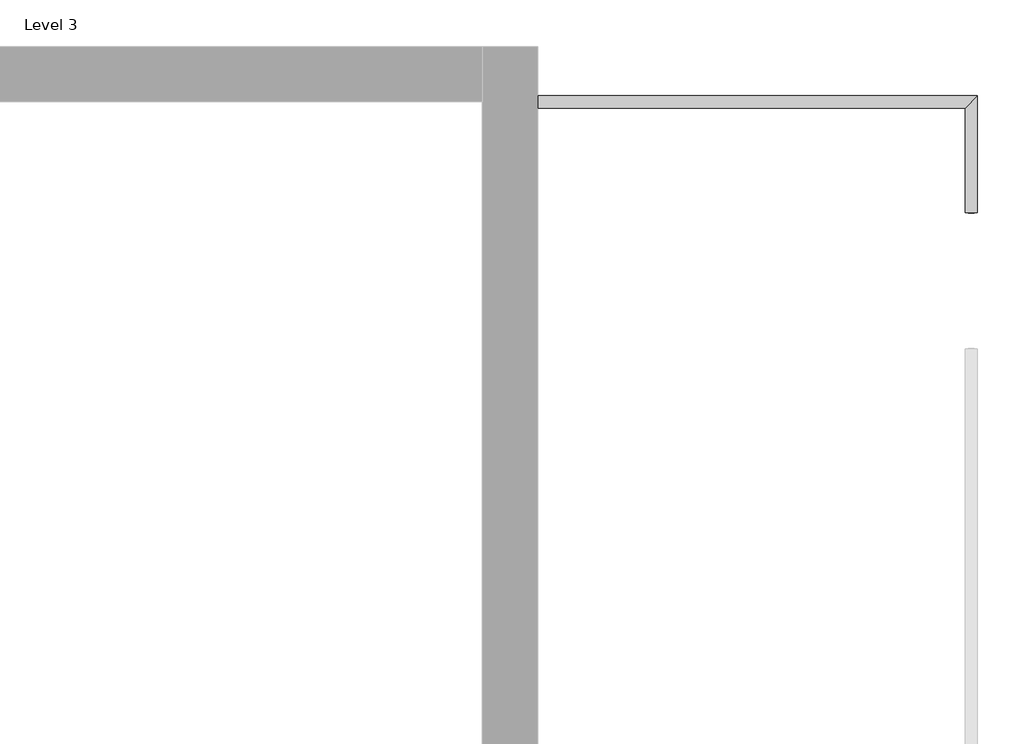
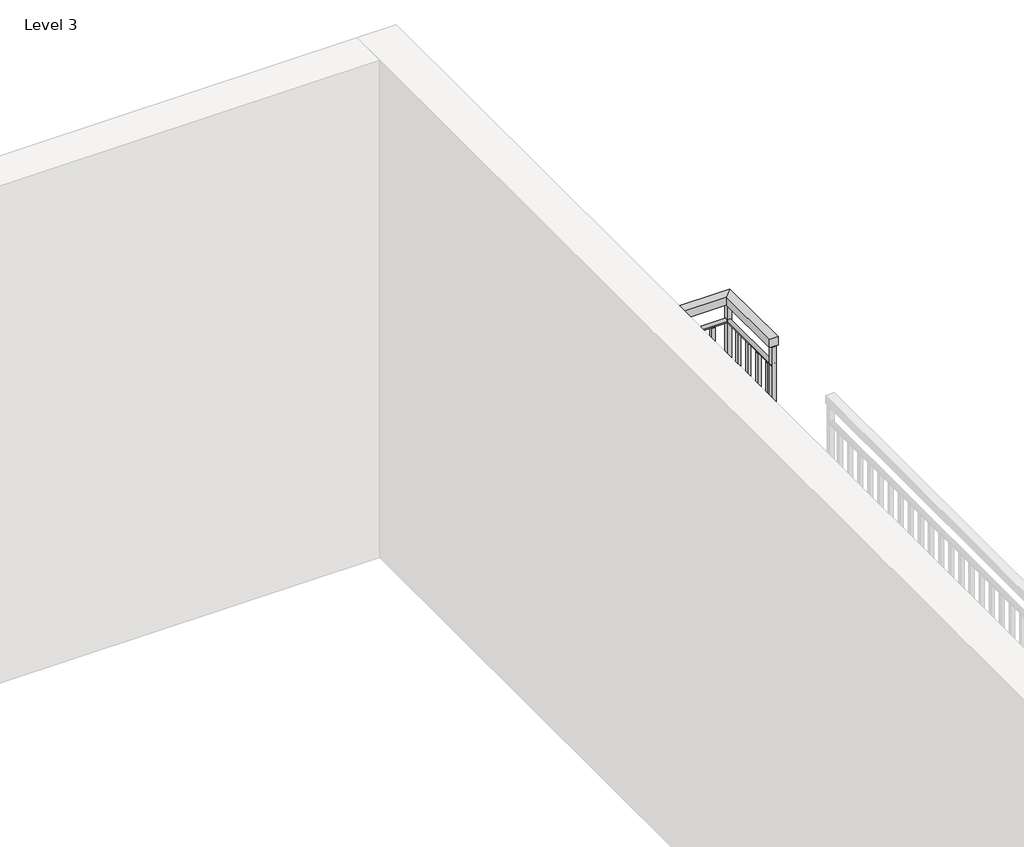
# One storey, part 4 of 4: 1 railing.
"""IFC4 building model written with IfcOpenShell, lengths in millimetres."""

from ifc_helpers import new_model, si_unit, frame, origin, place, context, project, spatial, polyline, circle_curve, ellipse_curve, outline, extrude, faceted_brep, element, save
from ifc_brep_helpers import plane_surface, cylinder_surface, advanced_brep

model = new_model("IFC4")

# Units and contexts
model_context = context("Model", 3, world=origin())
ifc_project = project(units=[si_unit("LENGTHUNIT", "METRE", prefix="MILLI")], contexts=[model_context])

# Site, building, storey
site = spatial("IfcSite", under=ifc_project)
building = spatial("IfcBuilding", under=site)
storey = spatial("IfcBuildingStorey", under=building, Name="Level 3", Elevation=3810.0)

# Railing
placement = place(None, origin())
element("IfcRailing", 1, ObjectType="Handrail - Rectangular", at=placement, inside=storey, context=model_context, shape_type="SolidModel", body=[
    faceted_brep([(6670.6750735, 9193.6050084, 4724.4), (6670.6750735, 9193.6050084, 4673.6), (6670.6750735, 9142.8050084, 4673.6), (6670.6750735, 9142.8050084, 4724.4), (8513.4425759, 9193.6050084, 4724.4), (8513.4425759, 9193.6050084, 4673.6), (8462.6425759, 9142.8050084, 4673.6), (8462.6425759, 9142.8050084, 4724.4), (8513.4425759, 8711.0050084, 4724.4), (8462.6425759, 8711.0050084, 4724.4), (8462.6425759, 8711.0050084, 4673.6), (8513.4425759, 8711.0050084, 4673.6)], [[[0, 1, 2, 3]], [[1, 0, 4, 5]], [[2, 1, 5, 6]], [[3, 2, 6, 7]], [[0, 3, 7, 4]], [[8, 9, 10, 11]], [[5, 4, 8, 11]], [[6, 5, 11, 10]], [[7, 6, 10, 9]], [[4, 7, 9, 8]]]),
    advanced_brep(
    [(6670.6750735, 9180.9050084, 4559.3), (6670.6750735, 9155.5050084, 4559.3), (8500.7425759, 9180.9050084, 4559.3), (8475.3425759, 9155.5050084, 4559.3), (8500.7425759, 8711.0050084, 4559.3), (8475.3425759, 8711.0050084, 4559.3)],
    [
        (0, 1, circle_curve(frame((6670.6750735, 9168.2050084, 4559.3), z_axis=(-1.0, 0.0, 0.0), x_axis=(0.0, -1.0, 0.0)), 12.7)),
        (1, 0, circle_curve(frame((6670.6750735, 9168.2050084, 4559.3), z_axis=(-1.0, 0.0, 0.0), x_axis=(0.0, -1.0, 0.0)), 12.7)),
        (0, 2),
        (2, 3, ellipse_curve(frame((8488.0425759, 9168.2050084, 4559.3), z_axis=(-0.7071067811865466, 0.7071067811865483, 0.0), x_axis=(-0.7071067811865486, -0.7071067811865466, 0.0)), 17.9605122, 12.7)),
        (3, 1),
        (3, 2, ellipse_curve(frame((8488.0425759, 9168.2050084, 4559.3), z_axis=(-0.7071067811865466, 0.7071067811865483, 0.0), x_axis=(-0.7071067811865486, -0.7071067811865466, 0.0)), 17.9605122, 12.7)),
        (4, 5, circle_curve(frame((8488.0425759, 8711.0050084, 4559.3), z_axis=(0.0, -1.0, 0.0), x_axis=(-1.0, 0.0, 0.0)), 12.7)),
        (5, 4, circle_curve(frame((8488.0425759, 8711.0050084, 4559.3), z_axis=(0.0, -1.0, 0.0), x_axis=(-1.0, 0.0, 0.0)), 12.7)),
        (2, 4),
        (5, 3),
    ],
    [
        plane_surface(frame((6670.6750735, 9168.2050084, 4572.0), z_axis=(-1.0, 0.0, 0.0), x_axis=(0.0, 1.0, 0.0))),
        cylinder_surface(frame((6670.6750735, 9168.2050084, 4559.3), z_axis=(-1.0, 0.0, 0.0), x_axis=(0.0, -1.0, 0.0)), 12.7),
        plane_surface(frame((8488.0425759, 8711.0050084, 4572.0), z_axis=(0.0, -1.0, 0.0), x_axis=(0.0, 0.0, -1.0))),
        cylinder_surface(frame((8488.0425759, 9168.2050084, 4559.3), z_axis=(0.0, 1.0, 0.0), x_axis=(-1.0, 0.0, 0.0)), 12.7),
    ],
    [
        (0, [[1, 2]]),
        (1, [[-1, 3, 4, 5]]),
        (1, [[-2, -5, 6, -3]]),
        (2, [[7, 8]]),
        (3, [[-4, 9, -8, 10]]),
        (3, [[-6, -10, -7, -9]]),
    ],
),
    advanced_brep(
    [(6670.6750735, 9180.9050084, 3949.7), (6670.6750735, 9155.5050084, 3949.7), (8500.7425759, 9180.9050084, 3949.7), (8475.3425759, 9155.5050084, 3949.7), (8500.7425759, 8711.0050084, 3949.7), (8475.3425759, 8711.0050084, 3949.7)],
    [
        (0, 1, circle_curve(frame((6670.6750735, 9168.2050084, 3949.7), z_axis=(-1.0, 0.0, 0.0), x_axis=(0.0, -1.0, 0.0)), 12.7)),
        (1, 0, circle_curve(frame((6670.6750735, 9168.2050084, 3949.7), z_axis=(-1.0, 0.0, 0.0), x_axis=(0.0, -1.0, 0.0)), 12.7)),
        (0, 2),
        (2, 3, ellipse_curve(frame((8488.0425759, 9168.2050084, 3949.7), z_axis=(-0.7071067811865466, 0.7071067811865483, 0.0), x_axis=(-0.7071067811865486, -0.7071067811865466, 0.0)), 17.9605122, 12.7)),
        (3, 1),
        (3, 2, ellipse_curve(frame((8488.0425759, 9168.2050084, 3949.7), z_axis=(-0.7071067811865466, 0.7071067811865483, 0.0), x_axis=(-0.7071067811865486, -0.7071067811865466, 0.0)), 17.9605122, 12.7)),
        (4, 5, circle_curve(frame((8488.0425759, 8711.0050084, 3949.7), z_axis=(0.0, -1.0, 0.0), x_axis=(-1.0, 0.0, 0.0)), 12.7)),
        (5, 4, circle_curve(frame((8488.0425759, 8711.0050084, 3949.7), z_axis=(0.0, -1.0, 0.0), x_axis=(-1.0, 0.0, 0.0)), 12.7)),
        (2, 4),
        (5, 3),
    ],
    [
        plane_surface(frame((6670.6750735, 9168.2050084, 3962.4), z_axis=(-1.0, 0.0, 0.0), x_axis=(0.0, 1.0, 0.0))),
        cylinder_surface(frame((6670.6750735, 9168.2050084, 3949.7), z_axis=(-1.0, 0.0, 0.0), x_axis=(0.0, -1.0, 0.0)), 12.7),
        plane_surface(frame((8488.0425759, 8711.0050084, 3962.4), z_axis=(0.0, -1.0, 0.0), x_axis=(0.0, 0.0, -1.0))),
        cylinder_surface(frame((8488.0425759, 9168.2050084, 3949.7), z_axis=(0.0, 1.0, 0.0), x_axis=(-1.0, 0.0, 0.0)), 12.7),
    ],
    [
        (0, [[1, 2]]),
        (1, [[-1, 3, 4, 5]]),
        (1, [[-2, -5, 6, -3]]),
        (2, [[7, 8]]),
        (3, [[-4, 9, -8, 10]]),
        (3, [[-6, -10, -7, -9]]),
    ],
),
    extrude(outline(polyline([(8478.5175759, 8771.3300084), (8497.5675759, 8771.3300084), (8497.5675759, 8752.2800084), (8478.5175759, 8752.2800084), (8478.5175759, 8771.3300084)])), frame((0.0, 0.0, 3810.0), z_axis=(0.0, 0.0, 1.0), x_axis=(1.0, 0.0, 0.0)), (0.0, 0.0, 1.0), 736.6),
    extrude(outline(polyline([(8478.5175759, 8872.9300084), (8497.5675759, 8872.9300084), (8497.5675759, 8853.8800084), (8478.5175759, 8853.8800084), (8478.5175759, 8872.9300084)])), frame((0.0, 0.0, 3810.0), z_axis=(0.0, 0.0, 1.0), x_axis=(1.0, 0.0, 0.0)), (0.0, 0.0, 1.0), 736.6),
    extrude(outline(polyline([(8478.5175759, 8974.5300084), (8497.5675759, 8974.5300084), (8497.5675759, 8955.4800084), (8478.5175759, 8955.4800084), (8478.5175759, 8974.5300084)])), frame((0.0, 0.0, 3810.0), z_axis=(0.0, 0.0, 1.0), x_axis=(1.0, 0.0, 0.0)), (0.0, 0.0, 1.0), 736.6),
    extrude(outline(polyline([(8478.5175759, 9076.1300084), (8497.5675759, 9076.1300084), (8497.5675759, 9057.0800084), (8478.5175759, 9057.0800084), (8478.5175759, 9076.1300084)])), frame((0.0, 0.0, 3810.0), z_axis=(0.0, 0.0, 1.0), x_axis=(1.0, 0.0, 0.0)), (0.0, 0.0, 1.0), 736.6),
    extrude(outline(polyline([(8388.3500735, 9158.6800084), (8388.3500735, 9177.7300084), (8407.4000735, 9177.7300084), (8407.4000735, 9158.6800084), (8388.3500735, 9158.6800084)])), frame((0.0, 0.0, 3810.0), z_axis=(0.0, 0.0, 1.0), x_axis=(1.0, 0.0, 0.0)), (0.0, 0.0, 1.0), 736.6),
    extrude(outline(polyline([(8286.7500735, 9158.6800084), (8286.7500735, 9177.7300084), (8305.8000735, 9177.7300084), (8305.8000735, 9158.6800084), (8286.7500735, 9158.6800084)])), frame((0.0, 0.0, 3810.0), z_axis=(0.0, 0.0, 1.0), x_axis=(1.0, 0.0, 0.0)), (0.0, 0.0, 1.0), 736.6),
    extrude(outline(polyline([(8185.1500735, 9158.6800084), (8185.1500735, 9177.7300084), (8204.2000735, 9177.7300084), (8204.2000735, 9158.6800084), (8185.1500735, 9158.6800084)])), frame((0.0, 0.0, 3810.0), z_axis=(0.0, 0.0, 1.0), x_axis=(1.0, 0.0, 0.0)), (0.0, 0.0, 1.0), 736.6),
    extrude(outline(polyline([(8083.5500735, 9158.6800084), (8083.5500735, 9177.7300084), (8102.6000735, 9177.7300084), (8102.6000735, 9158.6800084), (8083.5500735, 9158.6800084)])), frame((0.0, 0.0, 3810.0), z_axis=(0.0, 0.0, 1.0), x_axis=(1.0, 0.0, 0.0)), (0.0, 0.0, 1.0), 736.6),
    extrude(outline(polyline([(7981.9500735, 9158.6800084), (7981.9500735, 9177.7300084), (8001.0000735, 9177.7300084), (8001.0000735, 9158.6800084), (7981.9500735, 9158.6800084)])), frame((0.0, 0.0, 3810.0), z_axis=(0.0, 0.0, 1.0), x_axis=(1.0, 0.0, 0.0)), (0.0, 0.0, 1.0), 736.6),
    extrude(outline(polyline([(7880.3500735, 9158.6800084), (7880.3500735, 9177.7300084), (7899.4000735, 9177.7300084), (7899.4000735, 9158.6800084), (7880.3500735, 9158.6800084)])), frame((0.0, 0.0, 3810.0), z_axis=(0.0, 0.0, 1.0), x_axis=(1.0, 0.0, 0.0)), (0.0, 0.0, 1.0), 736.6),
    extrude(outline(polyline([(7778.7500735, 9158.6800084), (7778.7500735, 9177.7300084), (7797.8000735, 9177.7300084), (7797.8000735, 9158.6800084), (7778.7500735, 9158.6800084)])), frame((0.0, 0.0, 3810.0), z_axis=(0.0, 0.0, 1.0), x_axis=(1.0, 0.0, 0.0)), (0.0, 0.0, 1.0), 736.6),
    extrude(outline(polyline([(7677.1500735, 9158.6800084), (7677.1500735, 9177.7300084), (7696.2000735, 9177.7300084), (7696.2000735, 9158.6800084), (7677.1500735, 9158.6800084)])), frame((0.0, 0.0, 3810.0), z_axis=(0.0, 0.0, 1.0), x_axis=(1.0, 0.0, 0.0)), (0.0, 0.0, 1.0), 736.6),
    extrude(outline(polyline([(7575.5500735, 9158.6800084), (7575.5500735, 9177.7300084), (7594.6000735, 9177.7300084), (7594.6000735, 9158.6800084), (7575.5500735, 9158.6800084)])), frame((0.0, 0.0, 3810.0), z_axis=(0.0, 0.0, 1.0), x_axis=(1.0, 0.0, 0.0)), (0.0, 0.0, 1.0), 736.6),
    extrude(outline(polyline([(7473.9500735, 9158.6800084), (7473.9500735, 9177.7300084), (7493.0000735, 9177.7300084), (7493.0000735, 9158.6800084), (7473.9500735, 9158.6800084)])), frame((0.0, 0.0, 3810.0), z_axis=(0.0, 0.0, 1.0), x_axis=(1.0, 0.0, 0.0)), (0.0, 0.0, 1.0), 736.6),
    extrude(outline(polyline([(7372.3500735, 9158.6800084), (7372.3500735, 9177.7300084), (7391.4000735, 9177.7300084), (7391.4000735, 9158.6800084), (7372.3500735, 9158.6800084)])), frame((0.0, 0.0, 3810.0), z_axis=(0.0, 0.0, 1.0), x_axis=(1.0, 0.0, 0.0)), (0.0, 0.0, 1.0), 736.6),
    extrude(outline(polyline([(7270.7500735, 9158.6800084), (7270.7500735, 9177.7300084), (7289.8000735, 9177.7300084), (7289.8000735, 9158.6800084), (7270.7500735, 9158.6800084)])), frame((0.0, 0.0, 3810.0), z_axis=(0.0, 0.0, 1.0), x_axis=(1.0, 0.0, 0.0)), (0.0, 0.0, 1.0), 736.6),
    extrude(outline(polyline([(7169.1500735, 9158.6800084), (7169.1500735, 9177.7300084), (7188.2000735, 9177.7300084), (7188.2000735, 9158.6800084), (7169.1500735, 9158.6800084)])), frame((0.0, 0.0, 3810.0), z_axis=(0.0, 0.0, 1.0), x_axis=(1.0, 0.0, 0.0)), (0.0, 0.0, 1.0), 736.6),
    extrude(outline(polyline([(7067.5500735, 9158.6800084), (7067.5500735, 9177.7300084), (7086.6000735, 9177.7300084), (7086.6000735, 9158.6800084), (7067.5500735, 9158.6800084)])), frame((0.0, 0.0, 3810.0), z_axis=(0.0, 0.0, 1.0), x_axis=(1.0, 0.0, 0.0)), (0.0, 0.0, 1.0), 736.6),
    extrude(outline(polyline([(6965.9500735, 9158.6800084), (6965.9500735, 9177.7300084), (6985.0000735, 9177.7300084), (6985.0000735, 9158.6800084), (6965.9500735, 9158.6800084)])), frame((0.0, 0.0, 3810.0), z_axis=(0.0, 0.0, 1.0), x_axis=(1.0, 0.0, 0.0)), (0.0, 0.0, 1.0), 736.6),
    extrude(outline(polyline([(6864.3500735, 9158.6800084), (6864.3500735, 9177.7300084), (6883.4000735, 9177.7300084), (6883.4000735, 9158.6800084), (6864.3500735, 9158.6800084)])), frame((0.0, 0.0, 3810.0), z_axis=(0.0, 0.0, 1.0), x_axis=(1.0, 0.0, 0.0)), (0.0, 0.0, 1.0), 736.6),
    extrude(outline(polyline([(6762.7500735, 9158.6800084), (6762.7500735, 9177.7300084), (6781.8000735, 9177.7300084), (6781.8000735, 9158.6800084), (6762.7500735, 9158.6800084)])), frame((0.0, 0.0, 3810.0), z_axis=(0.0, 0.0, 1.0), x_axis=(1.0, 0.0, 0.0)), (0.0, 0.0, 1.0), 736.6),
    extrude(outline(polyline([(8475.3425759, 9155.5050084), (8475.3425759, 9180.9050084), (8500.7425759, 9180.9050084), (8500.7425759, 9155.5050084), (8475.3425759, 9155.5050084)])), frame((0.0, 0.0, 3810.0), z_axis=(0.0, 0.0, 1.0), x_axis=(1.0, 0.0, 0.0)), (0.0, 0.0, 1.0), 863.6),
    extrude(outline(polyline([(8475.3425759, 8733.2300084), (8500.7425759, 8733.2300084), (8500.7425759, 8707.8300084), (8475.3425759, 8707.8300084), (8475.3425759, 8733.2300084)])), frame((0.0, 0.0, 3810.0), z_axis=(0.0, 0.0, 1.0), x_axis=(1.0, 0.0, 0.0)), (0.0, 0.0, 1.0), 863.6),
    extrude(outline(polyline([(6667.5000735, 9155.5050084), (6667.5000735, 9180.9050084), (6692.9000735, 9180.9050084), (6692.9000735, 9155.5050084), (6667.5000735, 9155.5050084)])), frame((0.0, 0.0, 3810.0), z_axis=(0.0, 0.0, 1.0), x_axis=(1.0, 0.0, 0.0)), (0.0, 0.0, 1.0), 863.6),
])

save(model, "model.ifc")

# Revit data of these elements
# Type "Handrail - Rectangular"
#   Assembly Code = "C2010400"
#   built-in parameter 1008612 = 0.0416667 (stored number, unit not read)
#   built-in parameter 1008611 = 0.0416667 (stored number, unit not read)
#   built-in parameter 1008609 = 0.333333 (stored number, unit not read)
#   built-in parameter 1008604 = 0.166667 (stored number, unit not read)
#   built-in parameter 1008603 = 0.166667 (stored number, unit not read)
#   Railing Height = 3' - 0"
#   built-in parameter 1008630 = 2
#   built-in parameter 1008610 = 2
#   built-in parameter 1008618 = Baluster - Square : 3/4"
# Element 1 (IfcRailing, "Handrail - Rectangular")
#   Phase Created = New Construction
